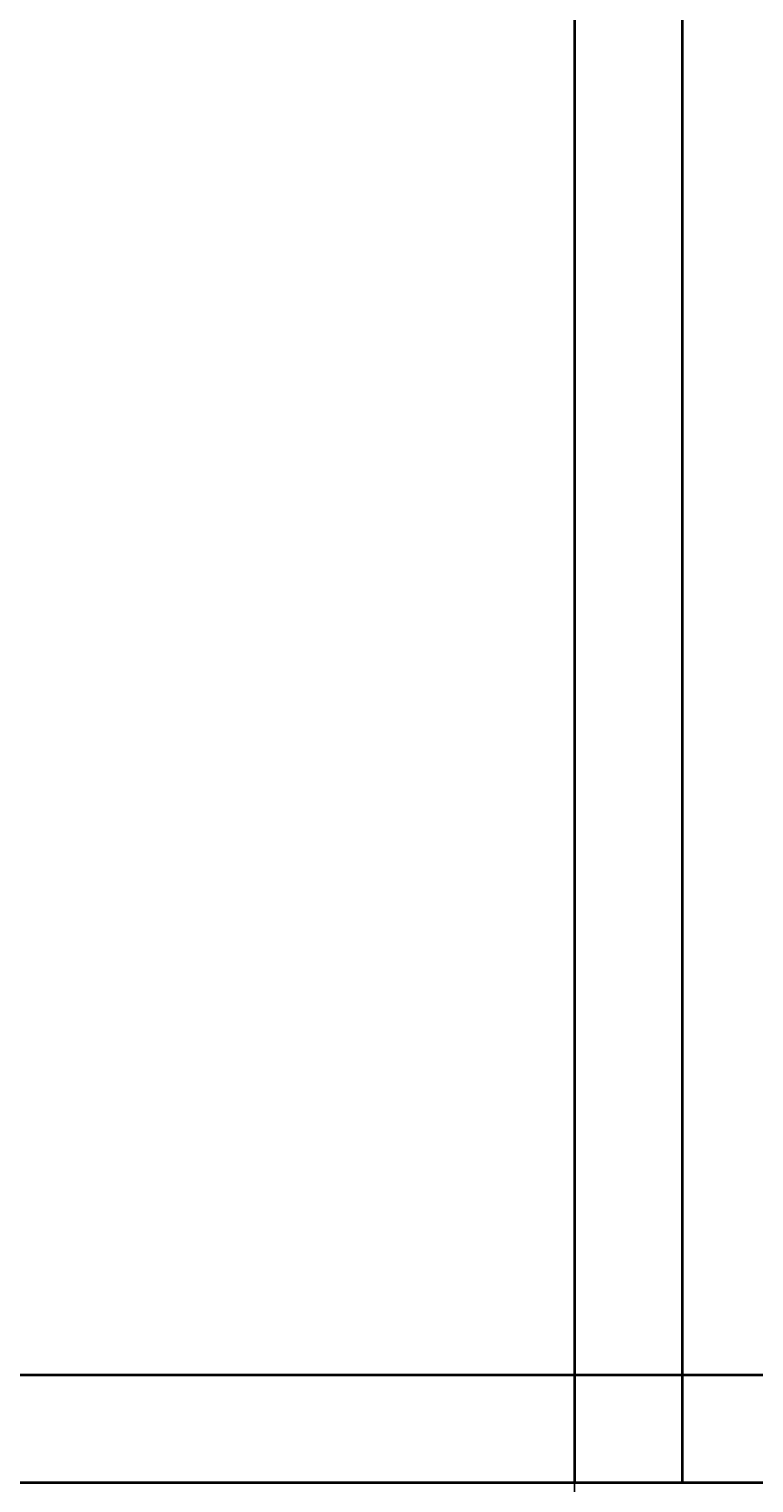
# Model space of a CAD drawing. Units: inches. Extents: x 867 to 1667, y -234 to 788.
# Tile 13 of 42: x 1151 to 1212, y 136 to 258. Entities that reach past the tile are written whole.
import ezdxf

# ---------------------------------------------------------------- set-up
doc = ezdxf.new("R2010")
doc.units = ezdxf.units.IN
doc.header["$MEASUREMENT"] = 0
doc.layers.add('A-ANNO-DIMS', color=2, linetype='Continuous', lineweight=18)
doc.layers.add('A-Wall', color=7, linetype='Continuous', lineweight=35)
doc.styles.get("Standard").update_dxf_attribs({"font": 'arial.ttf'})
doc.dimstyles.get("Standard").update_dxf_attribs({"dimtxt": 0.6875, "dimasz": 0.18, "dimexe": 0.18, "dimexo": 0.0625, "dimgap": 0.09, "dimtad": 0, "dimdec": 4, "dimzin": 0, "dimdsep": 46, "dimlunit": 4, "dimtxsty": 'Standard', "dimcen": 0.09, "dimadec": 0, "dimazin": 0, "dimtfac": 1, "dimtdec": 4, "dimtofl": 0, "dimtmove": 0, "dimatfit": 3, "dimfxl": 1, "dimtolj": 1, "dimtzin": 0, "dimarcsym": 0})

# ---------------------------------------------------------------- blocks, each defined once
blk = doc.blocks.new('*D37')
at = {"layer": 'A-ANNO-DIMS', "color": 0, "lineweight": -2, "transparency": 16777216}
for p, q in [((1049.89, 257.55), (1049.89, -233.54)), ((1196.89, 257.55), (1196.89, -233.54)), ((1050.07, -233.36), (1122.57, -233.36)), ((1196.71, -233.36), (1124.2, -233.36))]:
    blk.add_line(p, q, dxfattribs=at)
at = {"layer": 'A-ANNO-DIMS', "color": 0, "transparency": 16777216}
for points in [[(1050.07, -233.33), (1050.07, -233.39), (1049.89, -233.36)], [(1196.71, -233.33), (1196.71, -233.39), (1196.89, -233.36)]]:
    blk.add_solid(points, dxfattribs=at)
at = {"layer": 'Defpoints', "color": 0, "transparency": 16777216}
for p in [(1049.89, 257.62), (1196.89, 257.62), (1196.89, -233.36)]:
    blk.add_point(p, dxfattribs=at)
at = {"layer": 'A-ANNO-DIMS', "color": 0, "transparency": 16777216, "insert": (1123.39, -233.36), "char_height": 0.688, "attachment_point": 5}
blk.add_mtext('\\A1;147', dxfattribs=at)

msp = doc.modelspace()

# ---------------------------------------------------------------- linework, layer by layer
at = {"layer": 'A-Wall'}
for p, q in [((1196.8866, 404.617), (1196.8866, 136.117)), ((1205.8866, 404.617), (1205.8866, 136.117)), ((1301.3542, 145.117), (1070.8866, 145.117)), ((1301.3542, 136.117), (1070.8866, 136.117))]:
    msp.add_line(p, q, dxfattribs=at)

# ---------------------------------------------------------------- dimensions: what is measured, and where the dimension line sits
at = {"layer": 'A-ANNO-DIMS'}
dim = msp.add_linear_dim(base=(1196.8866, -233.3581), p1=(1049.8866, 257.617), p2=(1196.8866, 257.617), dimstyle='Standard', override={"dimdec": 0, "dimlfac": 1, "dimrnd": 0, "dimzin": 0, "dimdsep": 46, "dimlunit": 2}, dxfattribs=at)
dim.commit()
dim.dimension.update_dxf_attribs({"geometry": '*D37', "text_midpoint": (1123.3866, -233.3581)})

doc.saveas('drawing.dxf')
